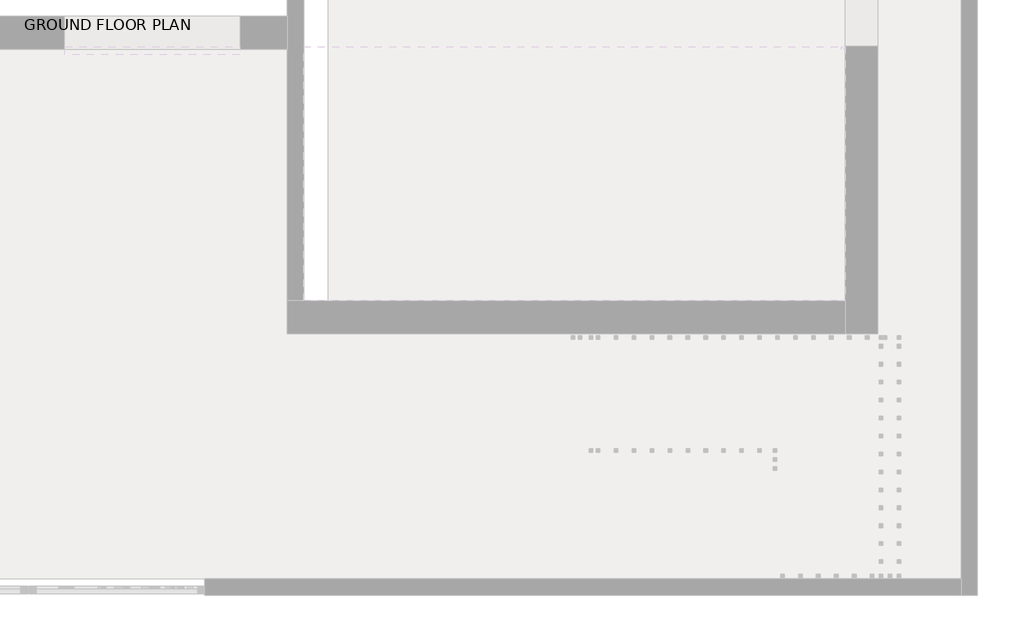
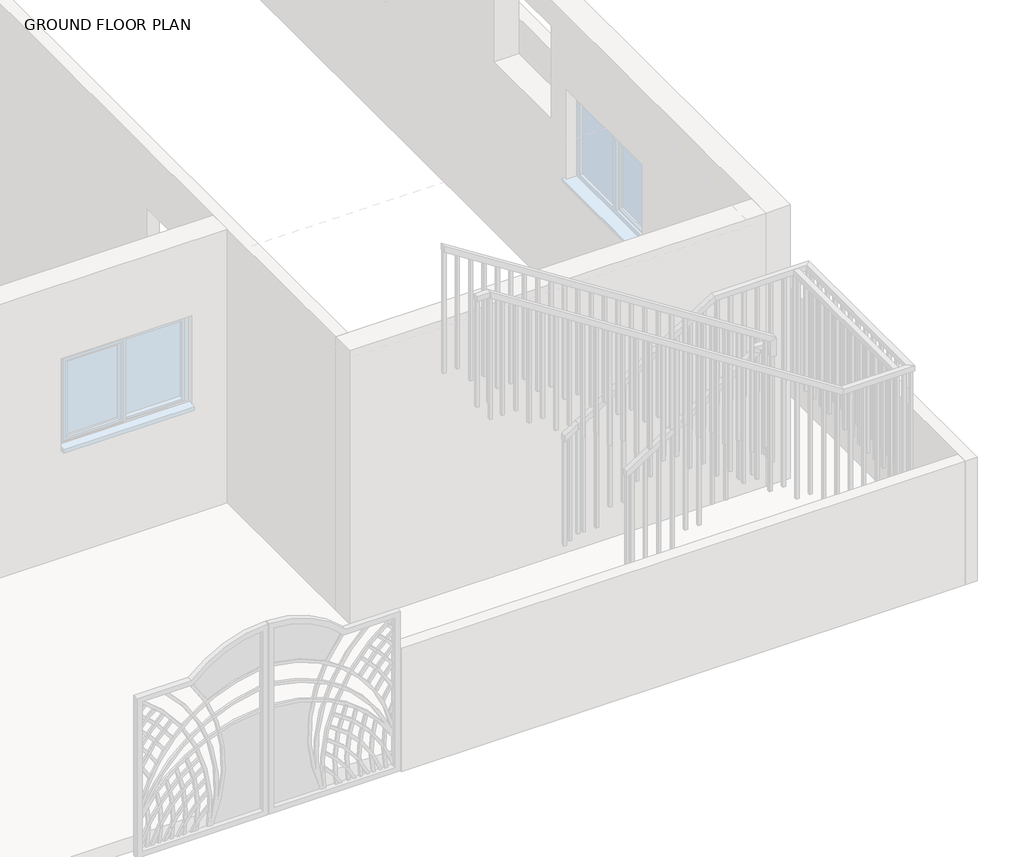
# One storey, part 9 of 23: 2 railings.
"""IFC4 building model written with IfcOpenShell, lengths in millimetres."""

from ifc_helpers import new_model, si_unit, frame, origin, place, context, project, spatial, polyline, outline, extrude, faceted_brep, element, save

model = new_model("IFC4")

# Units and contexts
model_context = context("Model", 3, world=origin())
ifc_project = project(units=[si_unit("LENGTHUNIT", "METRE", prefix="MILLI")], contexts=[model_context])

# Site, building, storey
site = spatial("IfcSite", under=ifc_project)
building = spatial("IfcBuilding", under=site)
storey = spatial("IfcBuildingStorey", under=building, Name="GROUND FLOOR PLAN", Elevation=487.68)

# Railings
placement = place(None, origin())
element("IfcRailing", 1, ObjectType="1100mm", at=placement, inside=storey, context=model_context, shape_type="SolidModel", body=[
    faceted_brep([(-8680.149573, -10220.0521308, 1912.8), (-8680.149573, -10220.0521308, 1853.4423995), (-8680.149573, -10270.0521308, 1853.4423995), (-8680.149573, -10270.0521308, 1912.8), (-7409.7306254, -10220.0521308, 2725.6), (-7395.1045513, -10220.0521308, 2675.6), (-7395.1045513, -10270.0521308, 2675.6), (-7409.7306254, -10270.0521308, 2725.6), (-6495.8132565, -10220.0521308, 2725.6), (-6495.8132565, -10220.0521308, 2675.6), (-6545.8132565, -10270.0521308, 2675.6), (-6545.8132565, -10270.0521308, 2725.6), (-6495.8132565, -11933.6860066, 2725.6), (-6495.8132565, -11933.6860066, 2675.6), (-6545.8132565, -11883.6860066, 2675.6), (-6545.8132565, -11883.6860066, 2725.6), (-7155.718398, -11933.6860066, 2725.6), (-7170.3479429, -11933.6860066, 2675.6), (-7170.3479429, -11883.6860066, 2675.6), (-7155.718398, -11883.6860066, 2725.6), (-10457.8773536, -11933.6860066, 4838.88), (-10457.8773536, -11883.6860066, 4838.88), (-10457.8773536, -11883.6860066, 4779.517542), (-10457.8773536, -11933.6860066, 4779.517542)], [[[0, 1, 2, 3]], [[1, 0, 4, 5]], [[2, 1, 5, 6]], [[3, 2, 6, 7]], [[0, 3, 7, 4]], [[5, 4, 8, 9]], [[6, 5, 9, 10]], [[7, 6, 10, 11]], [[4, 7, 11, 8]], [[9, 8, 12, 13]], [[10, 9, 13, 14]], [[11, 10, 14, 15]], [[8, 11, 15, 12]], [[13, 12, 16, 17]], [[14, 13, 17, 18]], [[15, 14, 18, 19]], [[12, 15, 19, 16]], [[20, 21, 22, 23]], [[17, 16, 20, 23]], [[18, 17, 23, 22]], [[19, 18, 22, 21]], [[16, 19, 21, 20]]]),
    extrude(outline(polyline([(4691.8007425, -10320.8132565), (4707.7999723, -10345.8132565), (3576.32, -10345.8132565), (3576.32, -10320.8132565), (4691.8007425, -10320.8132565)])), frame((0.0, -11921.1860066, 0.0), z_axis=(0.0, 1.0, 0.0), x_axis=(0.0, 0.0, 1.0)), (0.0, 0.0, 1.0), 25.0),
    extrude(outline(polyline([(4611.8045935, -10195.8132565), (4627.8038233, -10220.8132565), (3576.32, -10220.8132565), (3576.32, -10195.8132565), (4611.8045935, -10195.8132565)])), frame((0.0, -11921.1860066, 0.0), z_axis=(0.0, 1.0, 0.0), x_axis=(0.0, 0.0, 1.0)), (0.0, 0.0, 1.0), 25.0),
    extrude(outline(polyline([(4531.8084444, -10070.8132565), (4547.8076742, -10095.8132565), (3413.76, -10095.8132565), (3413.76, -10070.8132565), (4531.8084444, -10070.8132565)])), frame((0.0, -11921.1860066, 0.0), z_axis=(0.0, 1.0, 0.0), x_axis=(0.0, 0.0, 1.0)), (0.0, 0.0, 1.0), 25.0),
    extrude(outline(polyline([(4451.8122954, -9945.8132565), (4467.8115252, -9970.8132565), (3413.76, -9970.8132565), (3413.76, -9945.8132565), (4451.8122954, -9945.8132565)])), frame((0.0, -11921.1860066, 0.0), z_axis=(0.0, 1.0, 0.0), x_axis=(0.0, 0.0, 1.0)), (0.0, 0.0, 1.0), 25.0),
    extrude(outline(polyline([(4371.8161463, -9820.8132565), (4387.8153761, -9845.8132565), (3251.2, -9845.8132565), (3251.2, -9820.8132565), (4371.8161463, -9820.8132565)])), frame((0.0, -11921.1860066, 0.0), z_axis=(0.0, 1.0, 0.0), x_axis=(0.0, 0.0, 1.0)), (0.0, 0.0, 1.0), 25.0),
    extrude(outline(polyline([(4291.8423995, -9695.8132565), (4307.8371231, -9720.8132565), (3251.2, -9720.8132565), (3251.2, -9695.8132565), (4291.8423995, -9695.8132565)])), frame((0.0, -11921.1860066, 0.0), z_axis=(0.0, 1.0, 0.0), x_axis=(0.0, 0.0, 1.0)), (0.0, 0.0, 1.0), 25.0),
    extrude(outline(polyline([(4211.8238482, -9570.8132565), (4227.823078, -9595.8132565), (3088.64, -9595.8132565), (3088.64, -9570.8132565), (4211.8238482, -9570.8132565)])), frame((0.0, -11921.1860066, 0.0), z_axis=(0.0, 1.0, 0.0), x_axis=(0.0, 0.0, 1.0)), (0.0, 0.0, 1.0), 25.0),
    extrude(outline(polyline([(4131.8276992, -9445.8132565), (4147.826929, -9470.8132565), (3088.64, -9470.8132565), (3088.64, -9445.8132565), (4131.8276992, -9445.8132565)])), frame((0.0, -11921.1860066, 0.0), z_axis=(0.0, 1.0, 0.0), x_axis=(0.0, 0.0, 1.0)), (0.0, 0.0, 1.0), 25.0),
    extrude(outline(polyline([(4051.8315501, -9320.8132565), (4067.8307799, -9345.8132565), (2926.08, -9345.8132565), (2926.08, -9320.8132565), (4051.8315501, -9320.8132565)])), frame((0.0, -11921.1860066, 0.0), z_axis=(0.0, 1.0, 0.0), x_axis=(0.0, 0.0, 1.0)), (0.0, 0.0, 1.0), 25.0),
    extrude(outline(polyline([(3971.835401, -9195.8132565), (3987.8346309, -9220.8132565), (2926.08, -9220.8132565), (2926.08, -9195.8132565), (3971.835401, -9195.8132565)])), frame((0.0, -11921.1860066, 0.0), z_axis=(0.0, 1.0, 0.0), x_axis=(0.0, 0.0, 1.0)), (0.0, 0.0, 1.0), 25.0),
    extrude(outline(polyline([(3891.839252, -9070.8132565), (3907.8384818, -9095.8132565), (2763.52, -9095.8132565), (2763.52, -9070.8132565), (3891.839252, -9070.8132565)])), frame((0.0, -11921.1860066, 0.0), z_axis=(0.0, 1.0, 0.0), x_axis=(0.0, 0.0, 1.0)), (0.0, 0.0, 1.0), 25.0),
    extrude(outline(polyline([(3811.8431029, -8945.8132565), (3827.8423328, -8970.8132565), (2763.52, -8970.8132565), (2763.52, -8945.8132565), (3811.8431029, -8945.8132565)])), frame((0.0, -11921.1860066, 0.0), z_axis=(0.0, 1.0, 0.0), x_axis=(0.0, 0.0, 1.0)), (0.0, 0.0, 1.0), 25.0),
    extrude(outline(polyline([(3731.8469539, -8820.8132565), (3747.8461837, -8845.8132565), (2600.96, -8845.8132565), (2600.96, -8820.8132565), (3731.8469539, -8820.8132565)])), frame((0.0, -11921.1860066, 0.0), z_axis=(0.0, 1.0, 0.0), x_axis=(0.0, 0.0, 1.0)), (0.0, 0.0, 1.0), 25.0),
    extrude(outline(polyline([(3651.8508048, -8695.8132565), (3667.8500347, -8720.8132565), (2600.96, -8720.8132565), (2600.96, -8695.8132565), (3651.8508048, -8695.8132565)])), frame((0.0, -11921.1860066, 0.0), z_axis=(0.0, 1.0, 0.0), x_axis=(0.0, 0.0, 1.0)), (0.0, 0.0, 1.0), 25.0),
    extrude(outline(polyline([(3571.8546558, -8570.8132565), (3587.8538856, -8595.8132565), (2438.4, -8595.8132565), (2438.4, -8570.8132565), (3571.8546558, -8570.8132565)])), frame((0.0, -11921.1860066, 0.0), z_axis=(0.0, 1.0, 0.0), x_axis=(0.0, 0.0, 1.0)), (0.0, 0.0, 1.0), 25.0),
    extrude(outline(polyline([(3491.8585067, -8445.8132565), (3507.8577365, -8470.8132565), (2438.4, -8470.8132565), (2438.4, -8445.8132565), (3491.8585067, -8445.8132565)])), frame((0.0, -11921.1860066, 0.0), z_axis=(0.0, 1.0, 0.0), x_axis=(0.0, 0.0, 1.0)), (0.0, 0.0, 1.0), 25.0),
    extrude(outline(polyline([(3411.8623577, -8320.8132565), (3427.8615875, -8345.8132565), (2275.84, -8345.8132565), (2275.84, -8320.8132565), (3411.8623577, -8320.8132565)])), frame((0.0, -11921.1860066, 0.0), z_axis=(0.0, 1.0, 0.0), x_axis=(0.0, 0.0, 1.0)), (0.0, 0.0, 1.0), 25.0),
    extrude(outline(polyline([(3331.8662086, -8195.8132565), (3347.8654384, -8220.8132565), (2275.84, -8220.8132565), (2275.84, -8195.8132565), (3331.8662086, -8195.8132565)])), frame((0.0, -11921.1860066, 0.0), z_axis=(0.0, 1.0, 0.0), x_axis=(0.0, 0.0, 1.0)), (0.0, 0.0, 1.0), 25.0),
    extrude(outline(polyline([(3251.8700596, -8070.8132565), (3267.8692894, -8095.8132565), (2113.28, -8095.8132565), (2113.28, -8070.8132565), (3251.8700596, -8070.8132565)])), frame((0.0, -11921.1860066, 0.0), z_axis=(0.0, 1.0, 0.0), x_axis=(0.0, 0.0, 1.0)), (0.0, 0.0, 1.0), 25.0),
    extrude(outline(polyline([(3171.8739105, -7945.8132565), (3187.8731403, -7970.8132565), (2113.28, -7970.8132565), (2113.28, -7945.8132565), (3171.8739105, -7945.8132565)])), frame((0.0, -11921.1860066, 0.0), z_axis=(0.0, 1.0, 0.0), x_axis=(0.0, 0.0, 1.0)), (0.0, 0.0, 1.0), 25.0),
    extrude(outline(polyline([(3091.8777615, -7820.8132565), (3107.8769913, -7845.8132565), (1950.72, -7845.8132565), (1950.72, -7820.8132565), (3091.8777615, -7820.8132565)])), frame((0.0, -11921.1860066, 0.0), z_axis=(0.0, 1.0, 0.0), x_axis=(0.0, 0.0, 1.0)), (0.0, 0.0, 1.0), 25.0),
    extrude(outline(polyline([(3011.8816124, -7695.8132565), (3027.8808422, -7720.8132565), (1950.72, -7720.8132565), (1950.72, -7695.8132565), (3011.8816124, -7695.8132565)])), frame((0.0, -11921.1860066, 0.0), z_axis=(0.0, 1.0, 0.0), x_axis=(0.0, 0.0, 1.0)), (0.0, 0.0, 1.0), 25.0),
    extrude(outline(polyline([(2931.8854634, -7570.8132565), (2947.8846932, -7595.8132565), (1788.16, -7595.8132565), (1788.16, -7570.8132565), (2931.8854634, -7570.8132565)])), frame((0.0, -11921.1860066, 0.0), z_axis=(0.0, 1.0, 0.0), x_axis=(0.0, 0.0, 1.0)), (0.0, 0.0, 1.0), 25.0),
    extrude(outline(polyline([(2851.8893143, -7445.8132565), (2867.8885441, -7470.8132565), (1788.16, -7470.8132565), (1788.16, -7445.8132565), (2851.8893143, -7445.8132565)])), frame((0.0, -11921.1860066, 0.0), z_axis=(0.0, 1.0, 0.0), x_axis=(0.0, 0.0, 1.0)), (0.0, 0.0, 1.0), 25.0),
    extrude(outline(polyline([(2771.8931653, -7320.8132565), (2787.8923951, -7345.8132565), (1625.6, -7345.8132565), (1625.6, -7320.8132565), (2771.8931653, -7320.8132565)])), frame((0.0, -11921.1860066, 0.0), z_axis=(0.0, 1.0, 0.0), x_axis=(0.0, 0.0, 1.0)), (0.0, 0.0, 1.0), 25.0),
    extrude(outline(polyline([(2691.8970162, -7195.8132565), (2707.896246, -7220.8132565), (1625.6, -7220.8132565), (1625.6, -7195.8132565), (2691.8970162, -7195.8132565)])), frame((0.0, -11921.1860066, 0.0), z_axis=(0.0, 1.0, 0.0), x_axis=(0.0, 0.0, 1.0)), (0.0, 0.0, 1.0), 25.0),
    extrude(outline(polyline([(-7070.8132565, -11921.1860066), (-7095.8132565, -11921.1860066), (-7095.8132565, -11896.1860066), (-7070.8132565, -11896.1860066), (-7070.8132565, -11921.1860066)])), frame((0.0, 0.0, 1625.6), z_axis=(0.0, 0.0, 1.0), x_axis=(1.0, 0.0, 0.0)), (0.0, 0.0, 1.0), 1050.0),
    extrude(outline(polyline([(-6945.8132565, -11921.1860066), (-6970.8132565, -11921.1860066), (-6970.8132565, -11896.1860066), (-6945.8132565, -11896.1860066), (-6945.8132565, -11921.1860066)])), frame((0.0, 0.0, 1625.6), z_axis=(0.0, 0.0, 1.0), x_axis=(1.0, 0.0, 0.0)), (0.0, 0.0, 1.0), 1050.0),
    extrude(outline(polyline([(-6820.8132565, -11921.1860066), (-6845.8132565, -11921.1860066), (-6845.8132565, -11896.1860066), (-6820.8132565, -11896.1860066), (-6820.8132565, -11921.1860066)])), frame((0.0, 0.0, 1625.6), z_axis=(0.0, 0.0, 1.0), x_axis=(1.0, 0.0, 0.0)), (0.0, 0.0, 1.0), 1050.0),
    extrude(outline(polyline([(-6695.8132565, -11921.1860066), (-6720.8132565, -11921.1860066), (-6720.8132565, -11896.1860066), (-6695.8132565, -11896.1860066), (-6695.8132565, -11921.1860066)])), frame((0.0, 0.0, 1625.6), z_axis=(0.0, 0.0, 1.0), x_axis=(1.0, 0.0, 0.0)), (0.0, 0.0, 1.0), 1050.0),
    extrude(outline(polyline([(-6570.8132565, -11921.1860066), (-6595.8132565, -11921.1860066), (-6595.8132565, -11896.1860066), (-6570.8132565, -11896.1860066), (-6570.8132565, -11921.1860066)])), frame((0.0, 0.0, 1625.6), z_axis=(0.0, 0.0, 1.0), x_axis=(1.0, 0.0, 0.0)), (0.0, 0.0, 1.0), 1050.0),
    extrude(outline(polyline([(-6508.3132565, -11795.0521308), (-6508.3132565, -11820.0521308), (-6533.3132565, -11820.0521308), (-6533.3132565, -11795.0521308), (-6508.3132565, -11795.0521308)])), frame((0.0, 0.0, 1625.6), z_axis=(0.0, 0.0, 1.0), x_axis=(1.0, 0.0, 0.0)), (0.0, 0.0, 1.0), 1050.0),
    extrude(outline(polyline([(-6508.3132565, -11670.0521308), (-6508.3132565, -11695.0521308), (-6533.3132565, -11695.0521308), (-6533.3132565, -11670.0521308), (-6508.3132565, -11670.0521308)])), frame((0.0, 0.0, 1625.6), z_axis=(0.0, 0.0, 1.0), x_axis=(1.0, 0.0, 0.0)), (0.0, 0.0, 1.0), 1050.0),
    extrude(outline(polyline([(-6508.3132565, -11545.0521308), (-6508.3132565, -11570.0521308), (-6533.3132565, -11570.0521308), (-6533.3132565, -11545.0521308), (-6508.3132565, -11545.0521308)])), frame((0.0, 0.0, 1625.6), z_axis=(0.0, 0.0, 1.0), x_axis=(1.0, 0.0, 0.0)), (0.0, 0.0, 1.0), 1050.0),
    extrude(outline(polyline([(-6508.3132565, -11420.0521308), (-6508.3132565, -11445.0521308), (-6533.3132565, -11445.0521308), (-6533.3132565, -11420.0521308), (-6508.3132565, -11420.0521308)])), frame((0.0, 0.0, 1625.6), z_axis=(0.0, 0.0, 1.0), x_axis=(1.0, 0.0, 0.0)), (0.0, 0.0, 1.0), 1050.0),
    extrude(outline(polyline([(-6508.3132565, -11295.0521308), (-6508.3132565, -11320.0521308), (-6533.3132565, -11320.0521308), (-6533.3132565, -11295.0521308), (-6508.3132565, -11295.0521308)])), frame((0.0, 0.0, 1625.6), z_axis=(0.0, 0.0, 1.0), x_axis=(1.0, 0.0, 0.0)), (0.0, 0.0, 1.0), 1050.0),
    extrude(outline(polyline([(-6508.3132565, -11170.0521308), (-6508.3132565, -11195.0521308), (-6533.3132565, -11195.0521308), (-6533.3132565, -11170.0521308), (-6508.3132565, -11170.0521308)])), frame((0.0, 0.0, 1625.6), z_axis=(0.0, 0.0, 1.0), x_axis=(1.0, 0.0, 0.0)), (0.0, 0.0, 1.0), 1050.0),
    extrude(outline(polyline([(-6508.3132565, -11045.0521308), (-6508.3132565, -11070.0521308), (-6533.3132565, -11070.0521308), (-6533.3132565, -11045.0521308), (-6508.3132565, -11045.0521308)])), frame((0.0, 0.0, 1625.6), z_axis=(0.0, 0.0, 1.0), x_axis=(1.0, 0.0, 0.0)), (0.0, 0.0, 1.0), 1050.0),
    extrude(outline(polyline([(-6508.3132565, -10920.0521308), (-6508.3132565, -10945.0521308), (-6533.3132565, -10945.0521308), (-6533.3132565, -10920.0521308), (-6508.3132565, -10920.0521308)])), frame((0.0, 0.0, 1625.6), z_axis=(0.0, 0.0, 1.0), x_axis=(1.0, 0.0, 0.0)), (0.0, 0.0, 1.0), 1050.0),
    extrude(outline(polyline([(-6508.3132565, -10795.0521308), (-6508.3132565, -10820.0521308), (-6533.3132565, -10820.0521308), (-6533.3132565, -10795.0521308), (-6508.3132565, -10795.0521308)])), frame((0.0, 0.0, 1625.6), z_axis=(0.0, 0.0, 1.0), x_axis=(1.0, 0.0, 0.0)), (0.0, 0.0, 1.0), 1050.0),
    extrude(outline(polyline([(-6508.3132565, -10670.0521308), (-6508.3132565, -10695.0521308), (-6533.3132565, -10695.0521308), (-6533.3132565, -10670.0521308), (-6508.3132565, -10670.0521308)])), frame((0.0, 0.0, 1625.6), z_axis=(0.0, 0.0, 1.0), x_axis=(1.0, 0.0, 0.0)), (0.0, 0.0, 1.0), 1050.0),
    extrude(outline(polyline([(-6508.3132565, -10545.0521308), (-6508.3132565, -10570.0521308), (-6533.3132565, -10570.0521308), (-6533.3132565, -10545.0521308), (-6508.3132565, -10545.0521308)])), frame((0.0, 0.0, 1625.6), z_axis=(0.0, 0.0, 1.0), x_axis=(1.0, 0.0, 0.0)), (0.0, 0.0, 1.0), 1050.0),
    extrude(outline(polyline([(-6508.3132565, -10420.0521308), (-6508.3132565, -10445.0521308), (-6533.3132565, -10445.0521308), (-6533.3132565, -10420.0521308), (-6508.3132565, -10420.0521308)])), frame((0.0, 0.0, 1625.6), z_axis=(0.0, 0.0, 1.0), x_axis=(1.0, 0.0, 0.0)), (0.0, 0.0, 1.0), 1050.0),
    extrude(outline(polyline([(-6508.3132565, -10295.0521308), (-6508.3132565, -10320.0521308), (-6533.3132565, -10320.0521308), (-6533.3132565, -10295.0521308), (-6508.3132565, -10295.0521308)])), frame((0.0, 0.0, 1625.6), z_axis=(0.0, 0.0, 1.0), x_axis=(1.0, 0.0, 0.0)), (0.0, 0.0, 1.0), 1050.0),
    extrude(outline(polyline([(-6630.149573, -10232.5521308), (-6605.149573, -10232.5521308), (-6605.149573, -10257.5521308), (-6630.149573, -10257.5521308), (-6630.149573, -10232.5521308)])), frame((0.0, 0.0, 1625.6), z_axis=(0.0, 0.0, 1.0), x_axis=(1.0, 0.0, 0.0)), (0.0, 0.0, 1.0), 1050.0),
    extrude(outline(polyline([(-6755.149573, -10232.5521308), (-6730.149573, -10232.5521308), (-6730.149573, -10257.5521308), (-6755.149573, -10257.5521308), (-6755.149573, -10232.5521308)])), frame((0.0, 0.0, 1625.6), z_axis=(0.0, 0.0, 1.0), x_axis=(1.0, 0.0, 0.0)), (0.0, 0.0, 1.0), 1050.0),
    extrude(outline(polyline([(-6880.149573, -10232.5521308), (-6855.149573, -10232.5521308), (-6855.149573, -10257.5521308), (-6880.149573, -10257.5521308), (-6880.149573, -10232.5521308)])), frame((0.0, 0.0, 1625.6), z_axis=(0.0, 0.0, 1.0), x_axis=(1.0, 0.0, 0.0)), (0.0, 0.0, 1.0), 1050.0),
    extrude(outline(polyline([(-7005.149573, -10232.5521308), (-6980.149573, -10232.5521308), (-6980.149573, -10257.5521308), (-7005.149573, -10257.5521308), (-7005.149573, -10232.5521308)])), frame((0.0, 0.0, 1625.6), z_axis=(0.0, 0.0, 1.0), x_axis=(1.0, 0.0, 0.0)), (0.0, 0.0, 1.0), 1050.0),
    extrude(outline(polyline([(-7130.149573, -10232.5521308), (-7105.149573, -10232.5521308), (-7105.149573, -10257.5521308), (-7130.149573, -10257.5521308), (-7130.149573, -10232.5521308)])), frame((0.0, 0.0, 1625.6), z_axis=(0.0, 0.0, 1.0), x_axis=(1.0, 0.0, 0.0)), (0.0, 0.0, 1.0), 1050.0),
    extrude(outline(polyline([(-7255.149573, -10232.5521308), (-7230.149573, -10232.5521308), (-7230.149573, -10257.5521308), (-7255.149573, -10257.5521308), (-7255.149573, -10232.5521308)])), frame((0.0, 0.0, 1625.6), z_axis=(0.0, 0.0, 1.0), x_axis=(1.0, 0.0, 0.0)), (0.0, 0.0, 1.0), 1050.0),
    extrude(outline(polyline([(-7380.149573, -10232.5521308), (-7355.149573, -10232.5521308), (-7355.149573, -10257.5521308), (-7380.149573, -10257.5521308), (-7380.149573, -10232.5521308)])), frame((0.0, 0.0, 1625.6), z_axis=(0.0, 0.0, 1.0), x_axis=(1.0, 0.0, 0.0)), (0.0, 0.0, 1.0), 1050.0),
    extrude(outline(polyline([(1463.04, -7505.149573), (1463.04, -7480.149573), (2621.1891352, -7480.149573), (2605.1944115, -7505.149573), (1463.04, -7505.149573)])), frame((0.0, -10257.5521308, 0.0), z_axis=(0.0, 1.0, 0.0), x_axis=(0.0, 0.0, 1.0)), (0.0, 0.0, 1.0), 25.0),
    extrude(outline(polyline([(1463.04, -7630.149573), (1463.04, -7605.149573), (2541.2155169, -7605.149573), (2525.2207932, -7630.149573), (1463.04, -7630.149573)])), frame((0.0, -10257.5521308, 0.0), z_axis=(0.0, 1.0, 0.0), x_axis=(0.0, 0.0, 1.0)), (0.0, 0.0, 1.0), 25.0),
    extrude(outline(polyline([(1300.48, -7755.149573), (1300.48, -7730.149573), (2461.2418986, -7730.149573), (2445.2471749, -7755.149573), (1300.48, -7755.149573)])), frame((0.0, -10257.5521308, 0.0), z_axis=(0.0, 1.0, 0.0), x_axis=(0.0, 0.0, 1.0)), (0.0, 0.0, 1.0), 25.0),
    extrude(outline(polyline([(1300.48, -7880.149573), (1300.48, -7855.149573), (2381.2682803, -7855.149573), (2365.2735566, -7880.149573), (1300.48, -7880.149573)])), frame((0.0, -10257.5521308, 0.0), z_axis=(0.0, 1.0, 0.0), x_axis=(0.0, 0.0, 1.0)), (0.0, 0.0, 1.0), 25.0),
    extrude(outline(polyline([(1137.92, -8005.149573), (1137.92, -7980.149573), (2301.294662, -7980.149573), (2285.2999383, -8005.149573), (1137.92, -8005.149573)])), frame((0.0, -10257.5521308, 0.0), z_axis=(0.0, 1.0, 0.0), x_axis=(0.0, 0.0, 1.0)), (0.0, 0.0, 1.0), 25.0),
    extrude(outline(polyline([(1137.92, -8130.149573), (1137.92, -8105.149573), (2221.3210437, -8105.149573), (2205.32632, -8130.149573), (1137.92, -8130.149573)])), frame((0.0, -10257.5521308, 0.0), z_axis=(0.0, 1.0, 0.0), x_axis=(0.0, 0.0, 1.0)), (0.0, 0.0, 1.0), 25.0),
    extrude(outline(polyline([(975.36, -8255.149573), (975.36, -8230.149573), (2141.3474254, -8230.149573), (2125.3527017, -8255.149573), (975.36, -8255.149573)])), frame((0.0, -10257.5521308, 0.0), z_axis=(0.0, 1.0, 0.0), x_axis=(0.0, 0.0, 1.0)), (0.0, 0.0, 1.0), 25.0),
    extrude(outline(polyline([(975.36, -8380.149573), (975.36, -8355.149573), (2061.3738071, -8355.149573), (2045.3790834, -8380.149573), (975.36, -8380.149573)])), frame((0.0, -10257.5521308, 0.0), z_axis=(0.0, 1.0, 0.0), x_axis=(0.0, 0.0, 1.0)), (0.0, 0.0, 1.0), 25.0),
    extrude(outline(polyline([(812.8, -8505.149573), (812.8, -8480.149573), (1981.4001888, -8480.149573), (1965.4054651, -8505.149573), (812.8, -8505.149573)])), frame((0.0, -10257.5521308, 0.0), z_axis=(0.0, 1.0, 0.0), x_axis=(0.0, 0.0, 1.0)), (0.0, 0.0, 1.0), 25.0),
    extrude(outline(polyline([(812.8, -8630.149573), (812.8, -8605.149573), (1901.4265705, -8605.149573), (1885.4318468, -8630.149573), (812.8, -8630.149573)])), frame((0.0, -10257.5521308, 0.0), z_axis=(0.0, 1.0, 0.0), x_axis=(0.0, 0.0, 1.0)), (0.0, 0.0, 1.0), 25.0),
    extrude(outline(polyline([(-6508.3132565, -11896.1860066), (-6508.3132565, -11921.1860066), (-6533.3132565, -11921.1860066), (-6533.3132565, -11896.1860066), (-6508.3132565, -11896.1860066)])), frame((0.0, 0.0, 1625.6), z_axis=(0.0, 0.0, 1.0), x_axis=(1.0, 0.0, 0.0)), (0.0, 0.0, 1.0), 1050.0),
    extrude(outline(polyline([(-6533.3132565, -10232.5521308), (-6508.3132565, -10232.5521308), (-6508.3132565, -10257.5521308), (-6533.3132565, -10257.5521308), (-6533.3132565, -10232.5521308)])), frame((0.0, 0.0, 1625.6), z_axis=(0.0, 0.0, 1.0), x_axis=(1.0, 0.0, 0.0)), (0.0, 0.0, 1.0), 1050.0),
    extrude(outline(polyline([(4763.5183122, -10432.8773536), (4779.517542, -10457.8773536), (3576.32, -10457.8773536), (3576.32, -10432.8773536), (4763.5183122, -10432.8773536)])), frame((0.0, -11921.1860066, 0.0), z_axis=(0.0, 1.0, 0.0), x_axis=(0.0, 0.0, 1.0)), (0.0, 0.0, 1.0), 25.0),
    extrude(outline(polyline([(812.8, -8680.149573), (812.8, -8655.149573), (1869.4371231, -8655.149573), (1853.4423995, -8680.149573), (812.8, -8680.149573)])), frame((0.0, -10257.5521308, 0.0), z_axis=(0.0, 1.0, 0.0), x_axis=(0.0, 0.0, 1.0)), (0.0, 0.0, 1.0), 25.0),
])
element("IfcRailing", 2, ObjectType="1100mm", at=placement, inside=storey, context=model_context, shape_type="SolidModel", body=[
    faceted_brep([(-8680.149573, -11007.9255223, 1912.8), (-8680.149573, -11007.9255223, 1853.4423995), (-8680.149573, -11057.9255223, 1853.4423995), (-8680.149573, -11057.9255223, 1912.8), (-7484.3306254, -11007.9255223, 2677.8717446), (-7434.3306254, -11007.9255223, 2650.5035914), (-7434.3306254, -11057.9255223, 2650.5035914), (-7484.3306254, -11057.9255223, 2677.8717446), (-7484.3306254, -11007.9255223, 2725.6), (-7434.3306254, -11007.9255223, 2675.6), (-7434.3306254, -11057.9255223, 2675.6), (-7484.3306254, -11057.9255223, 2725.6), (-7359.3306254, -11007.9255223, 2725.6), (-7359.3306254, -11007.9255223, 2675.6), (-7409.3306254, -11057.9255223, 2675.6), (-7409.3306254, -11057.9255223, 2725.6), (-7359.3306254, -11132.9255223, 2725.6), (-7359.3306254, -11132.9255223, 2675.6), (-7409.3306254, -11132.9255223, 2675.6), (-7409.3306254, -11132.9255223, 2725.6), (-7359.3306254, -11134.9255223, 2725.6), (-7409.3306254, -11134.9255223, 2725.6), (-7409.3306254, -11184.9255223, 2675.6), (-7359.3306254, -11184.9255223, 2675.6)], [[[0, 1, 2, 3]], [[1, 0, 4, 5]], [[2, 1, 5, 6]], [[3, 2, 6, 7]], [[0, 3, 7, 4]], [[5, 4, 8, 9]], [[6, 5, 9, 10]], [[7, 6, 10, 11]], [[4, 7, 11, 8]], [[9, 8, 12, 13]], [[10, 9, 13, 14]], [[11, 10, 14, 15]], [[8, 11, 15, 12]], [[13, 12, 16, 17]], [[14, 13, 17, 18]], [[15, 14, 18, 19]], [[12, 15, 19, 16]], [[20, 21, 22, 23]], [[17, 16, 20, 23]], [[18, 17, 23, 22]], [[19, 18, 22, 21]], [[16, 19, 21, 20]]]),
    faceted_brep([(-7359.3306254, -11184.9255223, 2855.9055527), (-7409.3306254, -11184.9255223, 2828.5415543), (-7409.3306254, -11134.9255223, 2828.5415543), (-7359.3306254, -11134.9255223, 2855.9055527), (-10457.8773536, -11184.9255223, 4838.88), (-10457.8773536, -11134.9255223, 4838.88), (-10457.8773536, -11134.9255223, 4779.517542), (-10457.8773536, -11184.9255223, 4779.517542)], [[[0, 1, 2, 3]], [[4, 5, 6, 7]], [[1, 0, 4, 7]], [[2, 1, 7, 6]], [[3, 2, 6, 5]], [[0, 3, 5, 4]]]),
    faceted_brep([(-7359.3306254, -11134.9255223, 2725.6), (-7359.3306254, -11184.9255223, 2675.6), (-7409.3306254, -11184.9255223, 2675.6), (-7409.3306254, -11134.9255223, 2725.6), (-7359.3306254, -11134.9255223, 2855.9055527), (-7409.3306254, -11134.9255223, 2828.5415543), (-7409.3306254, -11184.9255223, 2828.5415543), (-7359.3306254, -11184.9255223, 2855.9055527)], [[[0, 1, 2, 3]], [[4, 5, 6, 7]], [[1, 0, 4, 7]], [[2, 1, 7, 6]], [[3, 2, 6, 5]], [[0, 3, 5, 4]]]),
    extrude(outline(polyline([(3576.32, -10434.3306254), (4764.4483614, -10434.3306254), (4780.4475912, -10459.3306254), (3576.32, -10459.3306254), (3576.32, -10434.3306254)])), frame((0.0, -11172.4255223, 0.0), z_axis=(0.0, 1.0, 0.0), x_axis=(0.0, 0.0, 1.0)), (0.0, 0.0, 1.0), 25.0),
    extrude(outline(polyline([(3576.32, -10309.3306254), (4684.4522123, -10309.3306254), (4700.4514422, -10334.3306254), (3576.32, -10334.3306254), (3576.32, -10309.3306254)])), frame((0.0, -11172.4255223, 0.0), z_axis=(0.0, 1.0, 0.0), x_axis=(0.0, 0.0, 1.0)), (0.0, 0.0, 1.0), 25.0),
    extrude(outline(polyline([(3413.76, -10184.3306254), (4604.4560633, -10184.3306254), (4620.4552931, -10209.3306254), (3413.76, -10209.3306254), (3413.76, -10184.3306254)])), frame((0.0, -11172.4255223, 0.0), z_axis=(0.0, 1.0, 0.0), x_axis=(0.0, 0.0, 1.0)), (0.0, 0.0, 1.0), 25.0),
    extrude(outline(polyline([(3413.76, -10059.3306254), (4524.4599142, -10059.3306254), (4540.459144, -10084.3306254), (3413.76, -10084.3306254), (3413.76, -10059.3306254)])), frame((0.0, -11172.4255223, 0.0), z_axis=(0.0, 1.0, 0.0), x_axis=(0.0, 0.0, 1.0)), (0.0, 0.0, 1.0), 25.0),
    extrude(outline(polyline([(3251.2, -9934.3306254), (4444.4637652, -9934.3306254), (4460.462995, -9959.3306254), (3251.2, -9959.3306254), (3251.2, -9934.3306254)])), frame((0.0, -11172.4255223, 0.0), z_axis=(0.0, 1.0, 0.0), x_axis=(0.0, 0.0, 1.0)), (0.0, 0.0, 1.0), 25.0),
    extrude(outline(polyline([(3251.2, -9809.3306254), (4364.4676161, -9809.3306254), (4380.4668459, -9834.3306254), (3251.2, -9834.3306254), (3251.2, -9809.3306254)])), frame((0.0, -11172.4255223, 0.0), z_axis=(0.0, 1.0, 0.0), x_axis=(0.0, 0.0, 1.0)), (0.0, 0.0, 1.0), 25.0),
    extrude(outline(polyline([(3251.2, -9684.3306254), (4284.4714671, -9684.3306254), (4300.4706969, -9709.3306254), (3251.2, -9709.3306254), (3251.2, -9684.3306254)])), frame((0.0, -11172.4255223, 0.0), z_axis=(0.0, 1.0, 0.0), x_axis=(0.0, 0.0, 1.0)), (0.0, 0.0, 1.0), 25.0),
    extrude(outline(polyline([(3088.64, -9559.3306254), (4204.475318, -9559.3306254), (4220.4745478, -9584.3306254), (3088.64, -9584.3306254), (3088.64, -9559.3306254)])), frame((0.0, -11172.4255223, 0.0), z_axis=(0.0, 1.0, 0.0), x_axis=(0.0, 0.0, 1.0)), (0.0, 0.0, 1.0), 25.0),
    extrude(outline(polyline([(3088.64, -9434.3306254), (4124.479169, -9434.3306254), (4140.4783988, -9459.3306254), (3088.64, -9459.3306254), (3088.64, -9434.3306254)])), frame((0.0, -11172.4255223, 0.0), z_axis=(0.0, 1.0, 0.0), x_axis=(0.0, 0.0, 1.0)), (0.0, 0.0, 1.0), 25.0),
    extrude(outline(polyline([(2926.08, -9309.3306254), (4044.4830199, -9309.3306254), (4060.4822497, -9334.3306254), (2926.08, -9334.3306254), (2926.08, -9309.3306254)])), frame((0.0, -11172.4255223, 0.0), z_axis=(0.0, 1.0, 0.0), x_axis=(0.0, 0.0, 1.0)), (0.0, 0.0, 1.0), 25.0),
    extrude(outline(polyline([(2926.08, -9184.3306254), (3964.4868709, -9184.3306254), (3980.4861007, -9209.3306254), (2926.08, -9209.3306254), (2926.08, -9184.3306254)])), frame((0.0, -11172.4255223, 0.0), z_axis=(0.0, 1.0, 0.0), x_axis=(0.0, 0.0, 1.0)), (0.0, 0.0, 1.0), 25.0),
    extrude(outline(polyline([(2763.52, -9059.3306254), (3884.4907218, -9059.3306254), (3900.4899516, -9084.3306254), (2763.52, -9084.3306254), (2763.52, -9059.3306254)])), frame((0.0, -11172.4255223, 0.0), z_axis=(0.0, 1.0, 0.0), x_axis=(0.0, 0.0, 1.0)), (0.0, 0.0, 1.0), 25.0),
    extrude(outline(polyline([(2763.52, -8934.3306254), (3804.4945728, -8934.3306254), (3820.4938026, -8959.3306254), (2763.52, -8959.3306254), (2763.52, -8934.3306254)])), frame((0.0, -11172.4255223, 0.0), z_axis=(0.0, 1.0, 0.0), x_axis=(0.0, 0.0, 1.0)), (0.0, 0.0, 1.0), 25.0),
    extrude(outline(polyline([(2600.96, -8809.3306254), (3724.4984237, -8809.3306254), (3740.4976535, -8834.3306254), (2600.96, -8834.3306254), (2600.96, -8809.3306254)])), frame((0.0, -11172.4255223, 0.0), z_axis=(0.0, 1.0, 0.0), x_axis=(0.0, 0.0, 1.0)), (0.0, 0.0, 1.0), 25.0),
    extrude(outline(polyline([(2600.96, -8684.3306254), (3644.5022747, -8684.3306254), (3660.5015045, -8709.3306254), (2600.96, -8709.3306254), (2600.96, -8684.3306254)])), frame((0.0, -11172.4255223, 0.0), z_axis=(0.0, 1.0, 0.0), x_axis=(0.0, 0.0, 1.0)), (0.0, 0.0, 1.0), 25.0),
    extrude(outline(polyline([(2438.4, -8559.3306254), (3564.5061256, -8559.3306254), (3580.5053554, -8584.3306254), (2438.4, -8584.3306254), (2438.4, -8559.3306254)])), frame((0.0, -11172.4255223, 0.0), z_axis=(0.0, 1.0, 0.0), x_axis=(0.0, 0.0, 1.0)), (0.0, 0.0, 1.0), 25.0),
    extrude(outline(polyline([(2438.4, -8434.3306254), (3484.5099766, -8434.3306254), (3500.5092064, -8459.3306254), (2438.4, -8459.3306254), (2438.4, -8434.3306254)])), frame((0.0, -11172.4255223, 0.0), z_axis=(0.0, 1.0, 0.0), x_axis=(0.0, 0.0, 1.0)), (0.0, 0.0, 1.0), 25.0),
    extrude(outline(polyline([(2275.84, -8309.3306254), (3404.5138275, -8309.3306254), (3420.5130573, -8334.3306254), (2275.84, -8334.3306254), (2275.84, -8309.3306254)])), frame((0.0, -11172.4255223, 0.0), z_axis=(0.0, 1.0, 0.0), x_axis=(0.0, 0.0, 1.0)), (0.0, 0.0, 1.0), 25.0),
    extrude(outline(polyline([(2275.84, -8184.3306254), (3324.5176785, -8184.3306254), (3340.5169083, -8209.3306254), (2275.84, -8209.3306254), (2275.84, -8184.3306254)])), frame((0.0, -11172.4255223, 0.0), z_axis=(0.0, 1.0, 0.0), x_axis=(0.0, 0.0, 1.0)), (0.0, 0.0, 1.0), 25.0),
    extrude(outline(polyline([(2113.28, -8059.3306254), (3244.5215294, -8059.3306254), (3260.5207592, -8084.3306254), (2113.28, -8084.3306254), (2113.28, -8059.3306254)])), frame((0.0, -11172.4255223, 0.0), z_axis=(0.0, 1.0, 0.0), x_axis=(0.0, 0.0, 1.0)), (0.0, 0.0, 1.0), 25.0),
    extrude(outline(polyline([(2113.28, -7934.3306254), (3164.5253804, -7934.3306254), (3180.5246102, -7959.3306254), (2113.28, -7959.3306254), (2113.28, -7934.3306254)])), frame((0.0, -11172.4255223, 0.0), z_axis=(0.0, 1.0, 0.0), x_axis=(0.0, 0.0, 1.0)), (0.0, 0.0, 1.0), 25.0),
    extrude(outline(polyline([(1950.72, -7809.3306254), (3084.5292313, -7809.3306254), (3100.5284611, -7834.3306254), (1950.72, -7834.3306254), (1950.72, -7809.3306254)])), frame((0.0, -11172.4255223, 0.0), z_axis=(0.0, 1.0, 0.0), x_axis=(0.0, 0.0, 1.0)), (0.0, 0.0, 1.0), 25.0),
    extrude(outline(polyline([(1950.72, -7684.3306254), (3004.5330823, -7684.3306254), (3020.5323121, -7709.3306254), (1950.72, -7709.3306254), (1950.72, -7684.3306254)])), frame((0.0, -11172.4255223, 0.0), z_axis=(0.0, 1.0, 0.0), x_axis=(0.0, 0.0, 1.0)), (0.0, 0.0, 1.0), 25.0),
    extrude(outline(polyline([(1788.16, -7559.3306254), (2924.5369332, -7559.3306254), (2940.536163, -7584.3306254), (1788.16, -7584.3306254), (1788.16, -7559.3306254)])), frame((0.0, -11172.4255223, 0.0), z_axis=(0.0, 1.0, 0.0), x_axis=(0.0, 0.0, 1.0)), (0.0, 0.0, 1.0), 25.0),
    extrude(outline(polyline([(1788.16, -7434.3306254), (2844.5407841, -7434.3306254), (2860.540014, -7459.3306254), (1788.16, -7459.3306254), (1788.16, -7434.3306254)])), frame((0.0, -11172.4255223, 0.0), z_axis=(0.0, 1.0, 0.0), x_axis=(0.0, 0.0, 1.0)), (0.0, 0.0, 1.0), 25.0),
    extrude(outline(polyline([(-7396.8306254, -11082.9255223), (-7371.8306254, -11082.9255223), (-7371.8306254, -11107.9255223), (-7396.8306254, -11107.9255223), (-7396.8306254, -11082.9255223)])), frame((0.0, 0.0, 1625.6), z_axis=(0.0, 0.0, 1.0), x_axis=(1.0, 0.0, 0.0)), (0.0, 0.0, 1.0), 1050.0),
    extrude(outline(polyline([(2605.1944115, -7505.149573), (1463.04, -7505.149573), (1463.04, -7480.149573), (2621.1891352, -7480.149573), (2605.1944115, -7505.149573)])), frame((0.0, -11045.4255223, 0.0), z_axis=(0.0, 1.0, 0.0), x_axis=(0.0, 0.0, 1.0)), (0.0, 0.0, 1.0), 25.0),
    extrude(outline(polyline([(2525.2207932, -7630.149573), (1463.04, -7630.149573), (1463.04, -7605.149573), (2541.2155169, -7605.149573), (2525.2207932, -7630.149573)])), frame((0.0, -11045.4255223, 0.0), z_axis=(0.0, 1.0, 0.0), x_axis=(0.0, 0.0, 1.0)), (0.0, 0.0, 1.0), 25.0),
    extrude(outline(polyline([(2445.2471749, -7755.149573), (1300.48, -7755.149573), (1300.48, -7730.149573), (2461.2418986, -7730.149573), (2445.2471749, -7755.149573)])), frame((0.0, -11045.4255223, 0.0), z_axis=(0.0, 1.0, 0.0), x_axis=(0.0, 0.0, 1.0)), (0.0, 0.0, 1.0), 25.0),
    extrude(outline(polyline([(2365.2735566, -7880.149573), (1300.48, -7880.149573), (1300.48, -7855.149573), (2381.2682803, -7855.149573), (2365.2735566, -7880.149573)])), frame((0.0, -11045.4255223, 0.0), z_axis=(0.0, 1.0, 0.0), x_axis=(0.0, 0.0, 1.0)), (0.0, 0.0, 1.0), 25.0),
    extrude(outline(polyline([(2285.2999383, -8005.149573), (1137.92, -8005.149573), (1137.92, -7980.149573), (2301.294662, -7980.149573), (2285.2999383, -8005.149573)])), frame((0.0, -11045.4255223, 0.0), z_axis=(0.0, 1.0, 0.0), x_axis=(0.0, 0.0, 1.0)), (0.0, 0.0, 1.0), 25.0),
    extrude(outline(polyline([(2205.32632, -8130.149573), (1137.92, -8130.149573), (1137.92, -8105.149573), (2221.3210437, -8105.149573), (2205.32632, -8130.149573)])), frame((0.0, -11045.4255223, 0.0), z_axis=(0.0, 1.0, 0.0), x_axis=(0.0, 0.0, 1.0)), (0.0, 0.0, 1.0), 25.0),
    extrude(outline(polyline([(2125.3527017, -8255.149573), (975.36, -8255.149573), (975.36, -8230.149573), (2141.3474254, -8230.149573), (2125.3527017, -8255.149573)])), frame((0.0, -11045.4255223, 0.0), z_axis=(0.0, 1.0, 0.0), x_axis=(0.0, 0.0, 1.0)), (0.0, 0.0, 1.0), 25.0),
    extrude(outline(polyline([(2045.3790834, -8380.149573), (975.36, -8380.149573), (975.36, -8355.149573), (2061.3738071, -8355.149573), (2045.3790834, -8380.149573)])), frame((0.0, -11045.4255223, 0.0), z_axis=(0.0, 1.0, 0.0), x_axis=(0.0, 0.0, 1.0)), (0.0, 0.0, 1.0), 25.0),
    extrude(outline(polyline([(1965.4054651, -8505.149573), (812.8, -8505.149573), (812.8, -8480.149573), (1981.4001888, -8480.149573), (1965.4054651, -8505.149573)])), frame((0.0, -11045.4255223, 0.0), z_axis=(0.0, 1.0, 0.0), x_axis=(0.0, 0.0, 1.0)), (0.0, 0.0, 1.0), 25.0),
    extrude(outline(polyline([(1885.4318468, -8630.149573), (812.8, -8630.149573), (812.8, -8605.149573), (1901.4265705, -8605.149573), (1885.4318468, -8630.149573)])), frame((0.0, -11045.4255223, 0.0), z_axis=(0.0, 1.0, 0.0), x_axis=(0.0, 0.0, 1.0)), (0.0, 0.0, 1.0), 25.0),
    extrude(outline(polyline([(-7396.8306254, -11147.4255223), (-7371.8306254, -11147.4255223), (-7371.8306254, -11172.4255223), (-7396.8306254, -11172.4255223), (-7396.8306254, -11147.4255223)])), frame((0.0, 0.0, 1625.6), z_axis=(0.0, 0.0, 1.0), x_axis=(1.0, 0.0, 0.0)), (0.0, 0.0, 1.0), 1050.0),
    extrude(outline(polyline([(-7396.8306254, -11045.4255223), (-7396.8306254, -11020.4255223), (-7371.8306254, -11020.4255223), (-7371.8306254, -11045.4255223), (-7396.8306254, -11045.4255223)])), frame((0.0, 0.0, 1625.6), z_axis=(0.0, 0.0, 1.0), x_axis=(1.0, 0.0, 0.0)), (0.0, 0.0, 1.0), 1050.0),
    extrude(outline(polyline([(3576.32, -10432.8773536), (4763.5183122, -10432.8773536), (4779.517542, -10457.8773536), (3576.32, -10457.8773536), (3576.32, -10432.8773536)])), frame((0.0, -11172.4255223, 0.0), z_axis=(0.0, 1.0, 0.0), x_axis=(0.0, 0.0, 1.0)), (0.0, 0.0, 1.0), 25.0),
    extrude(outline(polyline([(1853.4423995, -8680.149573), (812.8, -8680.149573), (812.8, -8655.149573), (1869.4371231, -8655.149573), (1853.4423995, -8680.149573)])), frame((0.0, -11045.4255223, 0.0), z_axis=(0.0, 1.0, 0.0), x_axis=(0.0, 0.0, 1.0)), (0.0, 0.0, 1.0), 25.0),
])

save(model, "model.ifc")

# Revit data of these elements
# Type "1100mm"
#   built-in parameter 1008612 = 0.019685 (stored number, unit not read)
#   built-in parameter 1008611 = 0.019685 (stored number, unit not read)
#   built-in parameter 1008609 = 0.902231 (stored number, unit not read)
#   built-in parameter 1008604 = 0.19685 (stored number, unit not read)
#   built-in parameter 1008603 = 0.164042 (stored number, unit not read)
#   Railing Height = 3.608924 ft
#   built-in parameter 1008630 = 2
#   built-in parameter 1008610 = 2
#   built-in parameter 1008608 = 1
#   built-in parameter 1008618 = Baluster_Square : 25mm
# Elements 1, 2 (IfcRailing, "1100mm")
#   Phase Created = New Construction
